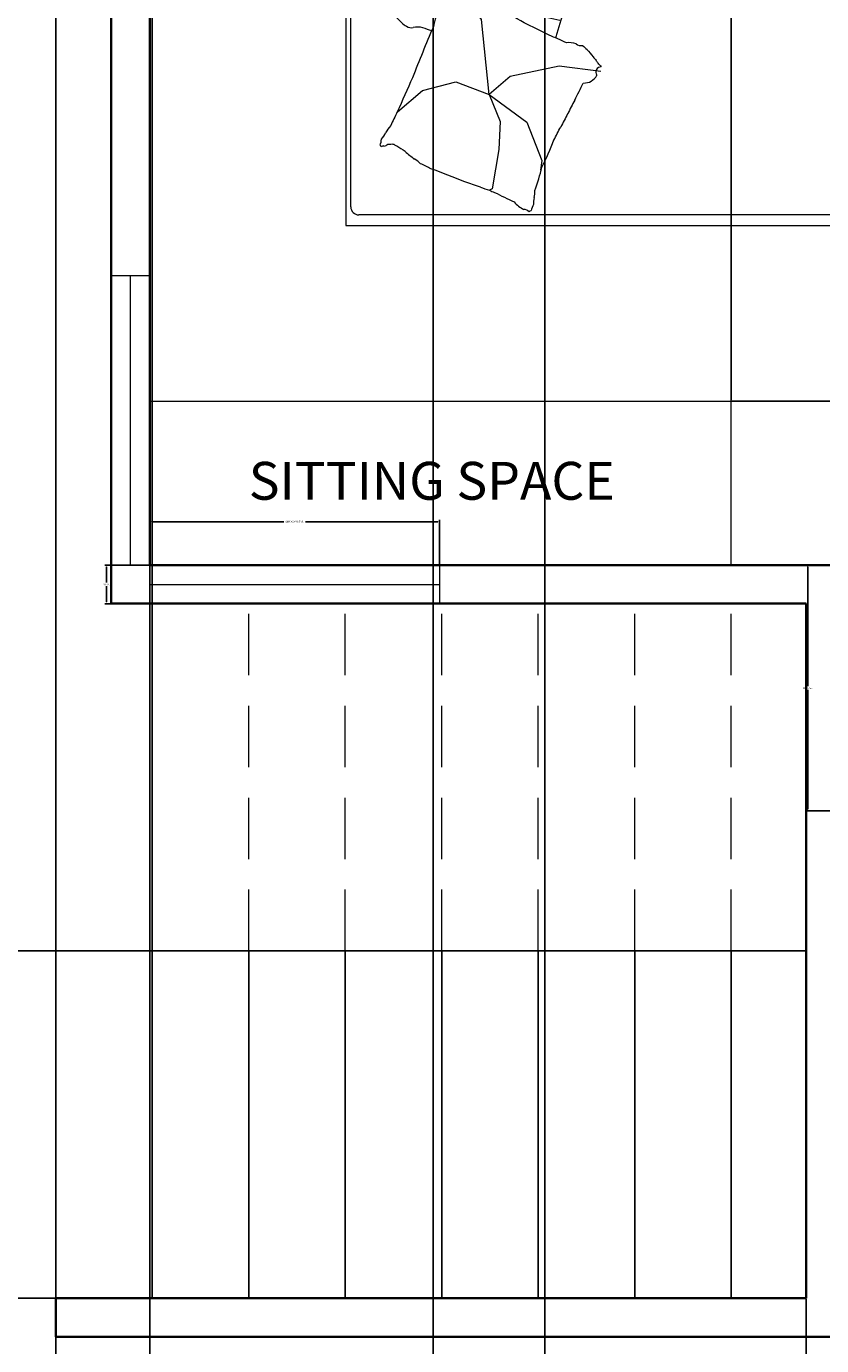
# Model space of a CAD drawing. Units: feet. Extents: x 1993 to 2298, y 2938 to 3641.
# Tile 3 of 11: x 2137 to 2219, y 3008 to 3144. Entities that reach past the tile are written whole.
import ezdxf

# ---------------------------------------------------------------- set-up
doc = ezdxf.new("R2010")
doc.units = ezdxf.units.FT
doc.linetypes.add('DASHED2', pattern=[9.525, 6.35, -3.175])
for name, color, linetype, lineweight in [('A-ANNO-DIMS', 2, 'Continuous', 18), ('A-AREA-IDEN', 7, 'Continuous', 18), ('A-FLOR-CASE', 8, 'Continuous', 18), ('A-FLOR-STRS', 7, 'Continuous', 25), ('A-FLOR-STRS-OVHD', 7, 'DASHED2', 13), ('A-GLAZ', 4, 'Continuous', 13), ('furniture', 8, 'Continuous', 18), ('WAL', 7, 'Continuous', 35)]:
    doc.layers.add(name, color=color, linetype=linetype, lineweight=lineweight)
doc.styles.add('DIM_FONT', font='SIMPLEX.shx', dxfattribs={"width": 0.8})
doc.styles.get("Standard").update_dxf_attribs({"font": 'arial.ttf'})
doc.dimstyles.get("Standard").update_dxf_attribs({"dimtxt": 0.18, "dimasz": 0.18, "dimexe": 0.18, "dimexo": 0.0625, "dimgap": 0.09, "dimtad": 0, "dimtih": 1, "dimtoh": 1, "dimdec": 4, "dimzin": 0, "dimdsep": 46, "dimtxsty": 'Standard', "dimcen": 0.09, "dimadec": 0, "dimazin": 0, "dimtfac": 1, "dimtdec": 4, "dimtofl": 0, "dimtmove": 0, "dimatfit": 3, "dimfxl": 1, "dimtolj": 1, "dimtzin": 0, "dimarcsym": 0})

# ---------------------------------------------------------------- blocks, each defined once
blk = doc.blocks.new('A$C79766A75')
for p, q in [((0.45, 1.9999), (0, 1.9999)), ((0, 1.9999), (0, 1.5499)), ((0.45, 1.5499), (0.45, 1.9999)), ((1.9506, 2), (0.4506, 2)), ((0.4506, 2), (0.4506, 0)), ((1.9506, 0), (1.9506, 2)), ((2.402, 1.9999), (1.952, 1.9999)), ((1.952, 1.9999), (1.952, 1.5499)), ((2.402, 1.5499), (2.402, 1.9999)), ((0.42, 1.9699), (0.03, 1.9699)), ((0.03, 1.9699), (0.03, 1.5799)), ((0.42, 1.5799), (0.42, 1.9699)), ((2.372, 1.9699), (1.982, 1.9699)), ((1.982, 1.9699), (1.982, 1.5799)), ((2.372, 1.5799), (2.372, 1.9699)), ((1.9506, 1.9476), (0.4506, 1.9476)), ((0.2304, 1.9125), (0.2304, 1.6061)), ((2.1824, 1.9125), (2.1824, 1.6061)), ((0.0743, 1.7595), (0.3834, 1.7595)), ((2.0263, 1.7595), (2.3354, 1.7595)), ((1.1461, 1.5617), (1.1254, 1.6443)), ((1.8553, 1.5617), (1.8346, 1.6443)), ((0.4234, 1.6034), (0.4228, 1.6034)), ((0.03, 1.5799), (0.42, 1.5799)), ((1.982, 1.5799), (2.372, 1.5799)), ((0, 1.5499), (0.45, 1.5499)), ((1.1536, 1.5317), (1.1461, 1.5617)), ((1.8628, 1.5317), (1.8553, 1.5617)), ((1.952, 1.5499), (2.402, 1.5499)), ((1.0972, 1.5115), (0.4791, 1.0841)), ((1.0972, 1.5115), (1.9048, 1.5115)), ((1.9248, 1.4915), (1.9248, 0.0322)), ((1.0383, 1.2184), (1.0246, 1.3138)), ((1.9048, 1.2389), (1.0354, 1.2389)), ((1.0365, 1.0883), (1.0383, 1.2184)), ((0.4791, 0.0622), (0.4791, 1.0841)), ((1.1731, 0.6316), (1.2523, 0.5276)), ((1.5696, 0.6317), (1.5559, 0.5286)), ((1.2523, 0.5276), (1.3274, 0.3973)), ((1.4223, 0.4407), (1.442, 0.5296)), ((1.5559, 0.5286), (1.5817, 0.4065)), ((1.6952, 0.4478), (1.7898, 0.4856)), ((1.7898, 0.4856), (1.8139, 0.4822)), ((1.4025, 0.3834), (1.4223, 0.4407)), ((1.6264, 0.355), (1.6952, 0.4478)), ((1.3274, 0.3973), (1.3452, 0.342)), ((1.5817, 0.4065), (1.6264, 0.355)), ((1.1139, 0.3597), (1.0779, 0.3397)), ((1.2167, 0.3736), (1.1139, 0.3597)), ((1.3452, 0.342), (1.2167, 0.3736)), ((1.3452, 0.342), (1.4025, 0.3834)), ((1.6264, 0.355), (1.6935, 0.3825)), ((1.6935, 0.3825), (1.7623, 0.379)), ((1.7623, 0.379), (1.8603, 0.3619)), ((1.8603, 0.3619), (1.8636, 0.3554)), ((1.2957, 0.2787), (1.3452, 0.342)), ((1.3452, 0.342), (1.3569, 0.2478)), ((1.4034, 0.3558), (1.3803, 0.2995)), ((1.4406, 0.3361), (1.3907, 0.3)), ((1.6264, 0.355), (1.4406, 0.3361)), ((1.5954, 0.2725), (1.6264, 0.355)), ((1.3803, 0.2995), (1.3626, 0.256)), ((1.3907, 0.3), (1.3787, 0.2914)), ((1.2305, 0.2313), (1.2957, 0.2787)), ((1.6161, 0.19), (1.5954, 0.2725)), ((1.1376, 0.2313), (1.2305, 0.2313)), ((1.3588, 0.2331), (1.3706, 0.1385)), ((1.6697, 0.1274), (1.6161, 0.19)), ((1.9048, 0.0122), (0.5291, 0.0122)), ((0.4506, 0), (1.9506, 0))]:
    blk.add_line(p, q)
for centre in [(0.2304, 1.7595), (2.1824, 1.7595)]:
    blk.add_circle(centre, 0.126)
for centre, radius, start, end in [((0.5232, 1.9139), 0.00342, 291.7883, 340.436), ((0.525, 1.9085), 0.00232, 340.436, 101.8931), ((0.5246, 1.9378), 0.0251, 274.3025, 291.7883), ((0.5311, 1.9093), 0.00428, 201.9904, 281.8931), ((0.5465, 1.8994), 0.0156, 158.579, 201.9904), ((0.5486, 1.9393), 0.0289, 239.3487, 274.3025), ((0.5458, 1.8568), 0.0539, 59.3487, 84.7408), ((0.546, 1.0829), 0.8208, 84.7408, 88.0921), ((0.6118, 2.0005), 0.0992, 254.0648, 274.2159), ((0.6775, 1.9817), 0.0992, 233.9136, 254.0648), ((0.6362, 0.406), 1.4943, 88.0921, 90.5757), ((0.7737, 2.1075), 0.234, 242.7604, 249.1397), ((0.7591, 1.0293), 0.8732, 90.5757, 94.8018), ((0.7631, 2.1919), 0.2897, 267.4614, 274.8018), ((0.8143, 2.0532), 0.1524, 259.8101, 267.4614), ((0.7515, 1.3747), 0.5293, 79.8101, 83.9133), ((1.1117, 1.6625), 0.2422, 97.5469, 105.744), ((1.0352, 2.2041), 0.3048, 278.4372, 285.744), ((1.1179, 2.0719), 0.1611, 270, 278.4372), ((1.1592, 2.0011), 0.0904, 258.7276, 270), ((1.1709, 1.9049), 0.0131, 153.4195, 258.7276), ((1.2325, 1.9139), 0.00342, 291.7883, 340.436), ((1.2342, 1.9085), 0.00232, 340.436, 101.8931), ((1.2338, 1.9378), 0.0251, 274.3025, 291.7883), ((1.2404, 1.9093), 0.00428, 201.9904, 281.8931), ((1.2558, 1.8994), 0.0156, 158.579, 201.9904), ((1.2578, 1.9393), 0.0289, 239.3487, 274.3025), ((1.2551, 1.8568), 0.0539, 59.3487, 84.7408), ((1.2552, 1.0829), 0.8208, 84.7408, 88.0921), ((1.3211, 2.0005), 0.0992, 254.0648, 274.2159), ((1.3868, 1.9817), 0.0992, 233.9136, 254.0648), ((1.3455, 0.406), 1.4943, 88.0921, 90.5757), ((1.4829, 2.1075), 0.234, 242.7604, 249.1397), ((1.4683, 1.0293), 0.8732, 90.5757, 94.8018), ((1.4724, 2.1919), 0.2897, 267.4614, 274.8018), ((1.5236, 2.0532), 0.1524, 259.8101, 267.4614), ((1.4607, 1.3747), 0.5293, 79.8101, 83.9133), ((1.821, 1.6625), 0.2422, 97.5469, 105.744), ((1.7444, 2.2041), 0.3048, 278.4372, 285.744), ((1.8271, 2.0719), 0.1611, 270, 278.4372), ((1.8684, 2.0011), 0.0904, 258.7276, 270), ((1.8802, 1.9049), 0.0131, 153.4195, 258.7276), ((0.4996, 1.8889), 0.0328, 338.579, 8.1335), ((0.2896, 1.8253), 0.246, 8.1335, 12.1095), ((0.7304, 1.9449), 0.0992, 216.1766, 233.9136), ((0.7661, 1.8961), 0.0992, 198.4397, 216.1766), ((0.738, 1.949), 0.0768, 231.6114, 242.7604), ((0.974, 2.1633), 0.3916, 226.1885, 231.6114), ((0.8451, 0.8466), 1.049, 83.9133, 90), ((1.046, 1.2129), 0.6827, 90, 97.5469), ((1.171, 1.8579), 0.0342, 94.4002, 153.4195), ((1.6324, 1.8735), 0.4918, 180, 186.2324), ((1.2088, 1.8889), 0.0328, 338.579, 8.1335), ((0.9988, 1.8253), 0.246, 8.1335, 12.1095), ((1.4396, 1.9449), 0.0992, 216.1766, 233.9136), ((1.4753, 1.8961), 0.0992, 198.4397, 216.1766), ((1.4473, 1.949), 0.0768, 231.6114, 242.7604), ((1.6833, 2.1633), 0.3916, 226.1885, 231.6114), ((1.5543, 0.8466), 1.049, 83.9133, 90), ((1.7552, 1.2129), 0.6827, 90, 97.5469), ((1.7511, 1.9723), 0.1399, 297.2036, 314.9024), ((1.8802, 1.8579), 0.0342, 94.4002, 153.4195), ((2.3416, 1.8735), 0.4918, 180, 186.2324), ((0.7297, 1.8867), 0.1983, 187.6809, 192.1095), ((1.4472, 1.8987), 0.9131, 183.3687, 187.6809), ((0.9057, 1.9982), 0.2252, 219.0349, 226.1885), ((0.7932, 1.8591), 0.0493, 208.3168, 219.0349), ((1.4389, 1.8867), 0.1983, 187.6809, 192.1095), ((2.1565, 1.8987), 0.9131, 183.3687, 187.6809), ((1.615, 1.9982), 0.2252, 219.0349, 226.1885), ((1.5025, 1.8591), 0.0493, 208.3168, 219.0349), ((1.6908, 1.9123), 0.1399, 314.9024, 332.6012), ((1.6887, 1.8881), 0.1511, 334.6449, 338.1851), ((1.7896, 1.8667), 0.0526, 318.5571, 334.6449), ((1.784, 1.9167), 0.0899, 306.2641, 318.5571), ((0.9392, 1.9062), 0.2002, 203.0028, 208.3168), ((1.3446, 1.7858), 0.204, 170.3156, 180), ((1.6484, 1.9062), 0.2002, 203.0028, 208.3168), ((1.6554, 1.8529), 0.1399, 332.6012, 343.485), ((1.7653, 1.8132), 0.0562, 341.2201, 0), ((1.6307, 1.8895), 0.2056, 338.1851, 341.2201), ((2.0538, 1.7858), 0.204, 170.3156, 180), ((1.2208, 1.7573), 0.6787, 178.3669, 183.3687), ((2.0027, 1.5994), 0.882, 167.8016, 170.3156), ((1.9301, 1.7573), 0.6787, 178.3669, 183.3687), ((1.6404, 1.8023), 0.1399, 343.485, 354.3689), ((1.73, 1.7719), 0.0915, 0, 14.6851), ((2.7119, 1.5994), 0.882, 167.8016, 170.3156), ((0.8192, 1.792), 0.3171, 347.8016, 351.9949), ((1.5284, 1.792), 0.3171, 347.8016, 351.9949), ((1.9066, 1.6447), 1.3652, 176.945, 178.3669), ((0.4711, 1.7556), 0.6588, 351.9949, 357.3351), ((2.6158, 1.6447), 1.3652, 176.945, 178.3669), ((1.1803, 1.7556), 0.6588, 351.9949, 357.3351), ((14.1519, 0.85), 13.6356, 176.49514, 176.94504), ((14.8612, 0.85), 13.6356, 176.49514, 176.94504), ((1.0578, 1.6474), 0.0677, 357.3351, 14.0452), ((1.767, 1.6474), 0.0677, 357.3351, 14.0452), ((0.7658, 2.8912), 1.4323, 294.3265, 296.4985), ((1.226, 2.0834), 0.5066, 290.6743, 294.3265), ((1.4305, 1.6796), 0.058, 274.0828, 290.6743), ((1.4679, 1.8969), 0.2721, 266.4448, 274.0828), ((0.8521, 1.5209), 0.3212, 170.0016, 176.4951), ((0.6583, 0.9067), 0.7387, 64.6889, 66.5156), ((0.7015, 0.888), 0.7387, 66.5156, 68.3423), ((1.5613, 1.5209), 0.3212, 170.0016, 176.4951), ((0.9025, 2.1618), 0.7286, 302.135, 305.8263), ((1.1895, 1.8508), 0.3126, 296.4985, 302.135), ((1.3675, 0.9067), 0.7387, 64.6889, 66.5156), ((1.4107, 0.888), 0.7387, 66.5156, 68.3423), ((0.513, 1.535), 0.0193, 350.0016, 16.6978), ((0.5822, 1.4654), 0.0767, 106.2212, 117.2841), ((0.5507, 1.5832), 0.0453, 282.869, 297.2841), ((0.5623, 1.6885), 0.1459, 273.574, 282.869), ((0.589, 2.7103), 1.164, 270.2865, 273.574), ((0.7584, 7.2662), 5.7185, 269.0296, 270.2865), ((0.9401, 4.9065), 3.3622, 267.3904, 269.0296), ((0.9811, 2.7573), 1.2165, 265.3824, 267.3904), ((0.8583, 0.139), 1.4048, 85.3824, 87.2509), ((1.0175, 1.3138), 0.2301, 87.2509, 101.5586), ((0.7501, 0.8688), 0.7387, 68.3423, 70.572), ((0.8043, 0.8497), 0.7387, 70.572, 72.8018), ((1.0449, 1.6886), 0.1459, 263.5659, 281.5586), ((1.1099, 1.6599), 0.1197, 252.6136, 263.5659), ((1.0587, 1.3144), 0.2297, 72.6136, 80.5159), ((1.2222, 1.535), 0.0193, 350.0016, 16.6978), ((1.2914, 1.4654), 0.0767, 106.2212, 117.2841), ((1.2599, 1.5832), 0.0453, 282.869, 297.2841), ((1.2716, 1.6885), 0.1459, 273.574, 282.869), ((1.2982, 2.7103), 1.164, 270.2865, 273.574), ((1.4677, 7.2662), 5.7185, 269.0296, 270.2865), ((1.6493, 4.9065), 3.3622, 267.3904, 269.0296), ((1.6903, 2.7573), 1.2165, 265.3824, 267.3904), ((1.5676, 0.139), 1.4048, 85.3824, 87.2509), ((1.7268, 1.3138), 0.2301, 87.2509, 101.5586), ((1.4594, 0.8688), 0.7387, 68.3423, 70.572), ((1.5136, 0.8497), 0.7387, 70.572, 72.8018), ((1.7541, 1.6886), 0.1459, 263.5659, 281.5586), ((1.8192, 1.6599), 0.1197, 252.6136, 263.5659), ((1.7679, 1.3144), 0.2297, 72.6136, 80.5159), ((0.5322, 1.5304), 0.00132, 16.6978, 97.1204), ((0.5579, 1.4467), 0.0875, 97.1204, 106.2212), ((0.745, 1.6407), 0.3751, 320.3555, 339.8512), ((1.108, 1.2635), 0.2708, 80.5159, 85.9171), ((1.1535, 1.5308), 0.000917, 85.9171, 194.0449), ((1.2414, 1.5304), 0.00132, 16.6978, 97.1204), ((1.2671, 1.4467), 0.0875, 97.1204, 106.2212), ((1.8172, 1.2635), 0.2708, 80.5159, 85.9171), ((1.8627, 1.5308), 0.000917, 85.9171, 194.0449), ((1.9048, 1.4915), 0.02, 0, 90), ((0.8556, 1.3759), 0.1801, 339.8512, 8.1356), ((1.9048, 1.2589), 0.02, 270, 0), ((-0.1888, 5.1029), 4.0646, 280.7276, 282.9255), ((0.7282, 1.1989), 0.0581, 262.2696, 280.7276), ((0.7833, 1.3309), 0.1942, 256.8096, 262.2696), ((0.2481, -1.3253), 2.5158, 76.8096, 78.3259), ((0.3953, -1.4284), 2.588, 78.3259, 80.505), ((-0.0248, 2.8487), 1.8351, 285.9352, 287.7364), ((0.3872, 1.7415), 0.6574, 282.9255, 285.9352), ((0.413, -2.64), 3.7801, 80.505, 82.308), ((1.1752, 0.6267), 0.0063, 166.7192, 233.4208), ((1.1734, 0.6272), 0.00443, 93.9484, 166.7192), ((1.163, 0.6103), 0.0142, 10.4074, 53.4208), ((1.1755, 0.5964), 0.0352, 69.6548, 93.9484), ((1.1669, 0.5731), 0.0601, 51.4146, 69.6548), ((1.7751, 0.3162), 0.3825, 126.2163, 127.5287), ((1.5806, 0.5924), 0.0452, 127.5287, 134.1274), ((1.5093, 0.6825), 0.0697, 308.8136, 314.1274), ((1.5706, 0.6318), 0.0127, 176.7545, 308.8136), ((1.5621, 0.59), 0.0359, 356.7545, 62.7098), ((0.8605, 0.749), 0.352, 329.0944, 333.1821), ((1.1396, 0.6079), 0.0393, 333.1821, 345.4291), ((1.1011, 0.5989), 0.0771, 2.7286, 10.4074), ((1.1628, 0.6019), 0.0153, 345.4291, 2.7286), ((1.2538, 0.682), 0.0792, 231.4146, 247.2931), ((1.5463, 1.3811), 0.8371, 247.2931, 249.8713), ((3.0113, 5.3783), 5.0942, 249.8713, 250.9164), ((1.4519, 0.6426), 0.0774, 313.5224, 324.1064), ((1.383, 0.7705), 0.2176, 307.2151, 313.5224), ((1.1426, 1.1456), 0.6605, 306.2163, 307.2151), ((0.9961, 0.6678), 0.194, 320.2995, 329.0944), ((2.374, 3.5362), 3.145, 250.9164, 253.3915), ((1.5435, 0.5526), 0.0458, 157.5838, 188.0492), ((1.4828, 0.5833), 0.0226, 324.1064, 8.0492), ((0.2201, -2.1858), 3.0972, 62.7098, 63.5853), ((2.5711, 2.3551), 2.0162, 242.5001, 243.5853), ((1.3115, 0.4414), 0.1965, 153.9265, 162.1604), ((1.2077, 0.4922), 0.081, 140.2995, 153.9265), ((2.4089, 0.1204), 1.0054, 154.9471, 157.5838), ((4.5245, 5.9445), 6.1019, 242.15178, 242.50014), ((-0.9881, -4.647), 5.8383, 62.15178, 62.50792), ((3.0311, -0.112), 2.003, 162.1604, 164.7375), ((2.9813, -0.2643), 1.6868, 152.9116, 154.9471), ((1.5084, 0.6341), 0.1166, 253.3915, 259.2634), ((1.5182, -0.068), 0.6236, 62.5079, 69.2514), ((1.7121, 0.0657), 0.43, 69.2514, 77.3748), ((1.8682, 0.4049), 0.063, 77.3748, 93.3881), ((1.8955, 0.5247), 0.0599, 256.9598, 273.3881), ((1.9257, 0.5082), 0.0509, 238.3083, 256.9598), ((1.9201, 0.4587), 0.0058, 180.9614, 238.3083), ((2.8096, -0.3311), 1.5652, 150.064, 152.9116), ((1.8435, 0.4743), 0.0755, 310.5086, 333.6668), ((1.9279, 0.441), 0.0168, 130.5086, 180.9614), ((2.6887, -0.0186), 1.6481, 164.7375, 166.159), ((-0.5166, 1.5491), 2.6619, 333.6668, 334.8268), ((0.5589, 0.5062), 0.5454, 343.6878, 346.159), ((1.2176, 0.4627), 0.2143, 330.064, 337.7645), ((1.701, 0.4319), 0.1798, 334.8268, 339.2919), ((-1.4109, 1.284), 2.6619, 338.0627, 339.2227), ((0.9098, 0.4035), 0.1798, 339.2227, 343.6878), ((3.4079, -0.2212), 1.6481, 160.3416, 161.7631), ((1.3456, 0.5261), 0.5454, 339.2919, 341.7631), ((3.6966, -0.4634), 2.003, 157.7645, 160.3416), ((1.0533, 0.2524), 0.0168, 134.9045, 185.3572), ((0.9882, 0.3177), 0.0755, 314.9045, 338.0627), ((1.0424, 0.2513), 0.0058, 185.3572, 242.7041), ((1.0631, 0.2914), 0.0509, 242.7041, 261.3557), ((1.0645, 0.3003), 0.0599, 261.3557, 277.784), ((1.0811, 0.1786), 0.063, 81.7707, 97.784), ((1.0286, -0.1846), 0.43, 73.6473, 81.7707), ((1.3465, 0.2383), 0.00467, 287.1867, 70.6201), ((1.3486, 0.2247), 0.0092, 70.6201, 94.2593), ((1.3694, 0.234), 0.0231, 107.1867, 157.7645), ((1.3563, 0.267), 0.034, 262.0178, 274.2593), ((1.4091, 0.4221), 0.1955, 255.1193, 262.0178), ((0.974, -0.3705), 0.6236, 66.9038, 73.6473), ((-1.0716, -5.1672), 5.8383, 66.54766, 66.9038), ((1.358, 0.0507), 0.1794, 75.1193, 82.3216), ((1.4096, 0.153), 0.0712, 82.3216, 94.5118), ((1.4285, 0.2893), 0.0663, 261.8784, 274.5118), ((1.4755, 0.332), 0.1166, 248.9957, 261.8784), ((2.7121, 3.1012), 3.145, 246.5205, 248.9957), ((2.4175, -0.1202), 1.0054, 160.6552, 161.9797), ((1.9797, 0.1108), 0.1965, 149.5306, 157.7645), ((3.6805, 5.7866), 6.1019, 246.54766, 246.89602), ((2.0773, 2.0287), 2.0162, 246.896, 247.9812), ((1.4382, 0.1619), 0.0226, 328.5023, 12.4451), ((1.505, 0.1766), 0.0458, 161.9797, 192.4451), ((3.6993, 4.7998), 5.0942, 245.4754, 246.5205), ((1.6279, 0.2819), 0.194, 315.9036, 324.6985), ((1.856, 0.1288), 0.081, 135.9036, 149.5306), ((0.1602, -2.7118), 3.0972, 67.1056, 67.9812), ((1.3512, 0.1084), 0.0359, 1.1504, 67.1056), ((1.2874, 0.2845), 0.2176, 311.611, 317.9183), ((1.3914, 0.1905), 0.0774, 317.9183, 328.5023), ((1.4661, 0.3294), 0.352, 324.6985, 328.7862), ((1.3997, 0.1094), 0.0127, 181.1504, 313.2095), ((1.3607, 0.1509), 0.0697, 313.2095, 318.5233), ((1.4468, 0.0748), 0.0452, 131.9246, 138.5233), ((1.6722, -0.1762), 0.3825, 130.6122, 131.9246), ((0.9933, 0.6156), 0.6605, 310.6122, 311.611), ((2.051, 0.8725), 0.8371, 242.8972, 245.4754), ((1.7576, 0.1689), 0.0792, 227.0187, 242.8972), ((1.6963, 0.0438), 0.0601, 47.0187, 65.2589), ((1.7345, 0.1188), 0.0153, 341.0332, 358.3327), ((1.6723, 0.1058), 0.0771, 358.3327, 6.0115), ((1.7401, 0.0928), 0.0142, 6.0115, 49.0249), ((1.7162, 0.1388), 0.0393, 328.7862, 341.0332), ((1.737, 0.0526), 0.0352, 65.2589, 89.5525), ((1.756, 0.0832), 0.00443, 89.5525, 162.3233), ((1.7602, 0.0924), 0.0063, 162.3233, 229.0249), ((0.5291, 0.0622), 0.05, 180, 270), ((1.9048, 0.0322), 0.02, 270, 0)]:
    blk.add_arc(centre, radius, start, end)
at = {"style": 'DIM_FONT', "text_generation_flag": 4, "width": 0.8, "flags": 9}
for tag in ['XSIZE', 'YSIZE']:
    blk.add_attdef(tag, (1.9506, 2), '', height=0.0005, rotation=180, dxfattribs=at)
blk = doc.blocks.new('WIN-2FT6')
for p, q in [((0, 4), (0, 0)), ((30, 4), (30, 0)), ((0, 2), (30, 2))]:
    blk.add_line(p, q)
blk = doc.blocks.new('*D28')
at = {"layer": 'A-ANNO-DIMS', "color": 0, "lineweight": -2, "transparency": 16777216}
for p, q in [((2221.7, 3088.53), (2217.75, 3088.53)), ((2217.93, 3088.35), (2217.93, 3075.97)), ((2217.93, 3063.22), (2217.93, 3075.6)), ((2221.7, 3063.04), (2217.75, 3063.04))]:
    blk.add_line(p, q, dxfattribs=at)
at = {"layer": 'A-ANNO-DIMS', "color": 0, "transparency": 16777216}
for points in [[(2217.9, 3088.35), (2217.96, 3088.35), (2217.93, 3088.53)], [(2217.9, 3063.22), (2217.96, 3063.22), (2217.93, 3063.04)]]:
    blk.add_solid(points, dxfattribs=at)
at = {"layer": 'Defpoints', "color": 0, "transparency": 16777216}
for p in [(2221.76, 3088.53), (2217.93, 3063.04), (2221.76, 3063.04)]:
    blk.add_point(p, dxfattribs=at)
at = {"layer": 'A-ANNO-DIMS', "color": 0, "transparency": 16777216, "insert": (2217.93, 3075.78), "char_height": 0.18, "attachment_point": 5}
blk.add_mtext('\\A1;DOOR 25', dxfattribs=at)
blk = doc.blocks.new('*D38')
at = {"layer": 'A-ANNO-DIMS', "color": 0, "lineweight": -2, "transparency": 16777216}
for p, q in [((2149.76, 3088.6), (2149.76, 3093.21)), ((2149.94, 3093.03), (2163.64, 3093.03)), ((2179.58, 3093.03), (2165.88, 3093.03)), ((2179.76, 3088.6), (2179.76, 3093.21))]:
    blk.add_line(p, q, dxfattribs=at)
at = {"layer": 'A-ANNO-DIMS', "color": 0, "transparency": 16777216}
for points in [[(2149.94, 3093.06), (2149.94, 3093), (2149.76, 3093.03)], [(2179.58, 3093.06), (2179.58, 3093), (2179.76, 3093.03)]]:
    blk.add_solid(points, dxfattribs=at)
at = {"layer": 'Defpoints', "color": 0, "transparency": 16777216}
for p in [(2179.76, 3093.03), (2149.76, 3088.53), (2179.76, 3088.53)]:
    blk.add_point(p, dxfattribs=at)
at = {"layer": 'A-ANNO-DIMS', "color": 0, "transparency": 16777216, "insert": (2164.76, 3093.03), "char_height": 0.18, "attachment_point": 5}
blk.add_mtext('\\A1;WINDOW 30 TYP.', dxfattribs=at)
blk = doc.blocks.new('*D39')
at = {"layer": 'A-ANNO-DIMS', "color": 0, "lineweight": -2, "transparency": 16777216}
for p, q in [((2149.7, 3088.53), (2145.08, 3088.53)), ((2145.26, 3088.35), (2145.26, 3086.71)), ((2145.26, 3084.71), (2145.26, 3086.35)), ((2149.7, 3084.53), (2145.08, 3084.53))]:
    blk.add_line(p, q, dxfattribs=at)
at = {"layer": 'A-ANNO-DIMS', "color": 0, "transparency": 16777216}
for points in [[(2145.23, 3088.35), (2145.29, 3088.35), (2145.26, 3088.53)], [(2145.23, 3084.71), (2145.29, 3084.71), (2145.26, 3084.53)]]:
    blk.add_solid(points, dxfattribs=at)
at = {"layer": 'Defpoints', "color": 0, "transparency": 16777216}
for p in [(2145.26, 3088.53), (2149.76, 3088.53), (2149.76, 3084.53)]:
    blk.add_point(p, dxfattribs=at)
at = {"layer": 'A-ANNO-DIMS', "color": 0, "transparency": 16777216, "insert": (2145.26, 3086.53), "char_height": 0.18, "attachment_point": 5}
blk.add_mtext('\\A1;4 TYP.', dxfattribs=at)
blk = doc.blocks.new('*D58')
at = {"layer": 'A-ANNO-DIMS', "color": 0, "lineweight": -2, "transparency": 16777216}
for p, q in [((2139.94, 3048.53), (1993.61, 3048.53)), ((1993.79, 3048.35), (1993.79, 3030.72)), ((1993.79, 3012.71), (1993.79, 3030.35)), ((2139.94, 3012.53), (1993.61, 3012.53))]:
    blk.add_line(p, q, dxfattribs=at)
at = {"layer": 'A-ANNO-DIMS', "color": 0, "transparency": 16777216}
for points in [[(1993.76, 3048.35), (1993.82, 3048.35), (1993.79, 3048.53)], [(1993.76, 3012.71), (1993.82, 3012.71), (1993.79, 3012.53)]]:
    blk.add_solid(points, dxfattribs=at)
at = {"layer": 'Defpoints', "color": 0, "transparency": 16777216}
for p in [(1993.79, 3048.53), (2140, 3048.53), (2140, 3012.53)]:
    blk.add_point(p, dxfattribs=at)
at = {"layer": 'A-ANNO-DIMS', "color": 0, "transparency": 16777216, "insert": (1993.79, 3030.53), "char_height": 0.18, "attachment_point": 5}
blk.add_mtext('\\A1;36', dxfattribs=at)
blk = doc.blocks.new('*D59')
at = {"layer": 'A-ANNO-DIMS', "color": 0, "lineweight": -2, "transparency": 16777216}
for p, q in [((2140, 3048.6), (2140, 3640.68)), ((2150, 3048.6), (2150, 3640.68)), ((2140.18, 3640.5), (2144.79, 3640.5)), ((2149.82, 3640.5), (2145.21, 3640.5))]:
    blk.add_line(p, q, dxfattribs=at)
at = {"layer": 'A-ANNO-DIMS', "color": 0, "transparency": 16777216}
for points in [[(2140.18, 3640.53), (2140.18, 3640.47), (2140, 3640.5)], [(2149.82, 3640.53), (2149.82, 3640.47), (2150, 3640.5)]]:
    blk.add_solid(points, dxfattribs=at)
at = {"layer": 'Defpoints', "color": 0, "transparency": 16777216}
for p in [(2150, 3640.5), (2140, 3048.53), (2150, 3048.53)]:
    blk.add_point(p, dxfattribs=at)
at = {"layer": 'A-ANNO-DIMS', "color": 0, "transparency": 16777216, "insert": (2145, 3640.5), "char_height": 0.18, "attachment_point": 5}
blk.add_mtext('\\A1;10', dxfattribs=at)
blk = doc.blocks.new('*D60')
at = {"layer": 'A-ANNO-DIMS', "color": 0, "lineweight": -2, "transparency": 16777216}
for p, q in [((2140, 3012.47), (2140, 2937.86)), ((2217.76, 3012.47), (2217.76, 2937.86)), ((2140.18, 2938.03), (2178.49, 2938.03)), ((2217.58, 2938.03), (2179.27, 2938.03))]:
    blk.add_line(p, q, dxfattribs=at)
at = {"layer": 'A-ANNO-DIMS', "color": 0, "transparency": 16777216}
for points in [[(2140.18, 2938.07), (2140.18, 2938.01), (2140, 2938.03)], [(2217.58, 2938.07), (2217.58, 2938.01), (2217.76, 2938.03)]]:
    blk.add_solid(points, dxfattribs=at)
at = {"layer": 'Defpoints', "color": 0, "transparency": 16777216}
for p in [(2140, 3012.53), (2217.76, 3012.53), (2217.76, 2938.03)]:
    blk.add_point(p, dxfattribs=at)
at = {"layer": 'A-ANNO-DIMS', "color": 0, "transparency": 16777216, "insert": (2178.88, 2938.03), "char_height": 0.18, "attachment_point": 5}
blk.add_mtext('\\A1;77.76', dxfattribs=at)
blk = doc.blocks.new('*D65')
at = {"layer": 'A-ANNO-DIMS', "color": 0, "lineweight": -2, "transparency": 16777216}
for p, q in [((2179.12, 3231.85), (2179.12, 2937.86)), ((2149.76, 3228.47), (2149.76, 2937.86)), ((2149.94, 2938.03), (2164.04, 2938.03)), ((2178.94, 2938.03), (2164.83, 2938.03))]:
    blk.add_line(p, q, dxfattribs=at)
at = {"layer": 'A-ANNO-DIMS', "color": 0, "transparency": 16777216}
for points in [[(2149.94, 2938.07), (2149.94, 2938.01), (2149.76, 2938.03)], [(2178.94, 2938.07), (2178.94, 2938.01), (2179.12, 2938.03)]]:
    blk.add_solid(points, dxfattribs=at)
at = {"layer": 'Defpoints', "color": 0, "transparency": 16777216}
for p in [(2179.12, 3231.92), (2149.76, 3228.53), (2179.12, 2938.03)]:
    blk.add_point(p, dxfattribs=at)
at = {"layer": 'A-ANNO-DIMS', "color": 0, "transparency": 16777216, "insert": (2164.44, 2938.03), "char_height": 0.18, "attachment_point": 5}
blk.add_mtext('\\A1;29.36', dxfattribs=at)
blk = doc.blocks.new('*D69')
at = {"layer": 'A-ANNO-DIMS', "color": 0, "lineweight": -2, "transparency": 16777216}
for p, q in [((2149.76, 3492.27), (2149.76, 2937.86)), ((2190.69, 3492.27), (2190.69, 2937.86)), ((2149.94, 2938.03), (2169.83, 2938.03)), ((2190.51, 2938.03), (2170.62, 2938.03))]:
    blk.add_line(p, q, dxfattribs=at)
at = {"layer": 'A-ANNO-DIMS', "color": 0, "transparency": 16777216}
for points in [[(2149.94, 2938.07), (2149.94, 2938.01), (2149.76, 2938.03)], [(2190.51, 2938.07), (2190.51, 2938.01), (2190.69, 2938.03)]]:
    blk.add_solid(points, dxfattribs=at)
at = {"layer": 'Defpoints', "color": 0, "transparency": 16777216}
for p in [(2149.76, 3492.33), (2190.69, 3492.33), (2190.69, 2938.03)]:
    blk.add_point(p, dxfattribs=at)
at = {"layer": 'A-ANNO-DIMS', "color": 0, "transparency": 16777216, "insert": (2170.23, 2938.03), "char_height": 0.18, "attachment_point": 5}
blk.add_mtext('\\A1;40.93', dxfattribs=at)
blk = doc.blocks.new('*D73')
at = {"layer": 'A-ANNO-DIMS', "color": 0, "lineweight": -2, "transparency": 16777216}
for p, q in [((2149.76, 3105.6), (2149.76, 3640.68)), ((2210, 3105.6), (2210, 3640.68)), ((2149.94, 3640.5), (2179.49, 3640.5)), ((2209.82, 3640.5), (2180.27, 3640.5))]:
    blk.add_line(p, q, dxfattribs=at)
at = {"layer": 'A-ANNO-DIMS', "color": 0, "transparency": 16777216}
for points in [[(2149.94, 3640.53), (2149.94, 3640.47), (2149.76, 3640.5)], [(2209.82, 3640.53), (2209.82, 3640.47), (2210, 3640.5)]]:
    blk.add_solid(points, dxfattribs=at)
at = {"layer": 'Defpoints', "color": 0, "transparency": 16777216}
for p in [(2210, 3640.5), (2149.76, 3105.53), (2210, 3105.53)]:
    blk.add_point(p, dxfattribs=at)
at = {"layer": 'A-ANNO-DIMS', "color": 0, "transparency": 16777216, "insert": (2179.88, 3640.5), "char_height": 0.18, "attachment_point": 5}
blk.add_mtext('\\A1;60.24', dxfattribs=at)
blk = doc.blocks.new('*D74')
at = {"layer": 'A-ANNO-DIMS', "color": 0, "lineweight": -2, "transparency": 16777216}
for p, q in [((2210.06, 3105.53), (2242.15, 3105.53)), ((2241.97, 3105.35), (2241.97, 3097.21)), ((2241.97, 3088.71), (2241.97, 3096.85)), ((2210.06, 3088.53), (2242.15, 3088.53))]:
    blk.add_line(p, q, dxfattribs=at)
at = {"layer": 'A-ANNO-DIMS', "color": 0, "transparency": 16777216}
for points in [[(2241.94, 3105.35), (2242, 3105.35), (2241.97, 3105.53)], [(2241.94, 3088.71), (2242, 3088.71), (2241.97, 3088.53)]]:
    blk.add_solid(points, dxfattribs=at)
at = {"layer": 'Defpoints', "color": 0, "transparency": 16777216}
for p in [(2210, 3105.53), (2210, 3088.53), (2241.97, 3088.53)]:
    blk.add_point(p, dxfattribs=at)
at = {"layer": 'A-ANNO-DIMS', "color": 0, "transparency": 16777216, "insert": (2241.97, 3097.03), "char_height": 0.18, "attachment_point": 5}
blk.add_mtext('\\A1;17', dxfattribs=at)
blk = doc.blocks.new('*D75')
at = {"layer": 'A-ANNO-DIMS', "color": 0, "lineweight": -2, "transparency": 16777216}
for p, q in [((2029.76, 3008.6), (2029.76, 3640.68)), ((2140, 3008.6), (2140, 3640.68)), ((2029.94, 3640.5), (2084.42, 3640.5)), ((2139.82, 3640.5), (2085.33, 3640.5))]:
    blk.add_line(p, q, dxfattribs=at)
at = {"layer": 'A-ANNO-DIMS', "color": 0, "transparency": 16777216}
for points in [[(2029.94, 3640.53), (2029.94, 3640.47), (2029.76, 3640.5)], [(2139.82, 3640.53), (2139.82, 3640.47), (2140, 3640.5)]]:
    blk.add_solid(points, dxfattribs=at)
at = {"layer": 'Defpoints', "color": 0, "transparency": 16777216}
for p in [(2140, 3640.5), (2029.76, 3008.53), (2140, 3008.53)]:
    blk.add_point(p, dxfattribs=at)
at = {"layer": 'A-ANNO-DIMS', "color": 0, "transparency": 16777216, "insert": (2084.88, 3640.5), "char_height": 0.18, "attachment_point": 5}
blk.add_mtext('\\A1;110.24', dxfattribs=at)

msp = doc.modelspace()

# ---------------------------------------------------------------- linework, layer by layer
at = {"layer": 'A-FLOR-CASE'}
for p in [(2149.7583, 3105.5338), (2210, 3088.5338)]:
    msp.add_line(p, (2210, 3105.5338), dxfattribs=at)
at = {"layer": 'A-FLOR-STRS'}
for p, q in [((2217.7583, 3048.5338), (2140, 3048.5338)), ((2140, 3048.5338), (2140, 3010.5338)), ((2150, 3048.5338), (2150, 3012.5338)), ((2160, 3048.5338), (2160, 3012.5338)), ((2170, 3048.5338), (2170, 3012.5338)), ((2180, 3048.5338), (2180, 3012.5338)), ((2190, 3048.5338), (2190, 3012.5338)), ((2200, 3048.5338), (2200, 3012.5338)), ((2210, 3048.5338), (2210, 3012.5338))]:
    msp.add_line(p, q, dxfattribs=at)
at = {"layer": 'A-FLOR-STRS-OVHD'}
for p, q in [((2150, 3048.5338), (2150, 3084.5338)), ((2160, 3048.5338), (2160, 3084.5338)), ((2170, 3048.5338), (2170, 3084.5338)), ((2180, 3048.5338), (2180, 3084.5338)), ((2190, 3048.5338), (2190, 3084.5338)), ((2200, 3048.5338), (2200, 3084.5338)), ((2210, 3048.5338), (2210, 3084.5338))]:
    msp.add_line(p, q, dxfattribs=at)
at = {"layer": 'WAL'}
for p, q in [((2145.7583, 3084.5338), (2145.7583, 3292.5338)), ((2149.7583, 3088.5338), (2149.7583, 3224.5338)), ((2149.7583, 3088.5338), (2221.7583, 3088.5338)), ((2145.7583, 3084.5338), (2217.7583, 3084.5338)), ((2217.7583, 3084.5338), (2217.7583, 3012.5338)), ((2217.7583, 3012.5338), (2140, 3012.5338)), ((2140, 3012.5338), (2140, 3008.5338)), ((2265.7583, 3008.5338), (2140, 3008.5338))]:
    msp.add_line(p, q, dxfattribs=at)

# ---------------------------------------------------------------- block references
at = {"layer": 'A-GLAZ', "rotation": 90.00000000000003}
msp.add_blockref('WIN-2FT6', (2149.7581, 3088.5335), dxfattribs=at)
at = {"layer": 'A-GLAZ'}
msp.add_blockref('WIN-2FT6', (2149.758, 3084.534), dxfattribs=at)
at = {"layer": 'furniture', "xscale": 41.83725109546206, "yscale": 41.83725109546206, "zscale": 41.83725109546206, "rotation": 270}
msp.add_blockref('A$C79766A75', (2170.0686, 3205.3572), dxfattribs=at)

# ---------------------------------------------------------------- texts
at = {"layer": 'A-AREA-IDEN'}
msp.add_text('SITTING SPACE', height=3.928054, dxfattribs=at).set_placement((2160, 3095.3045))

# ---------------------------------------------------------------- dimensions: what is measured, and where the dimension line sits
at = {"layer": 'A-ANNO-DIMS'}
for base, p1, p2, override, picture, middle in [((2140, 3640.4988), (2029.7583, 3008.5338), (2140, 3008.5338), {"dimdec": 2, "dimlfac": 1, "dimrnd": 0, "dimzin": 0, "dimdsep": 46, "dimlunit": 2}, '*D75', (2084.8792, 3640.4988)), ((2150, 3640.4988), (2140, 3048.5338), (2150, 3048.5338), {"dimdec": 0, "dimlfac": 1, "dimrnd": 0, "dimzin": 0, "dimdsep": 46, "dimlunit": 2}, '*D59', (2145, 3640.4988)), ((2210, 3640.4988), (2149.7583, 3105.5338), (2210, 3105.5338), {"dimdec": 2, "dimlfac": 1, "dimrnd": 0, "dimzin": 0, "dimdsep": 46, "dimlunit": 2}, '*D73', (2179.8792, 3640.4988)), ((2190.6917, 2938.035), (2149.7583, 3492.3338), (2190.6917, 3492.3338), {"dimdec": 2, "dimlfac": 1, "dimrnd": 0, "dimzin": 0, "dimdsep": 46, "dimlunit": 2}, '*D69', (2170.225, 2938.035)), ((2179.1188, 2938.035), (2149.7583, 3228.5338), (2179.1188, 3231.9167), {"dimdec": 2, "dimlfac": 1, "dimrnd": 0, "dimzin": 0, "dimdsep": 46, "dimlunit": 2}, '*D65', (2164.4386, 2938.035)), ((2217.7583, 2938.035), (2140, 3012.5338), (2217.7583, 3012.5338), {"dimdec": 2, "dimlfac": 1, "dimrnd": 0, "dimzin": 0, "dimdsep": 46, "dimlunit": 2}, '*D60', (2178.8792, 2938.035))]:
    dim = msp.add_linear_dim(base=base, p1=p1, p2=p2, dimstyle='Standard', override=override, dxfattribs=at)
    dim.commit()
    dim.dimension.update_dxf_attribs({"geometry": picture, "text_midpoint": middle})
for base, p1, p2, angle, picture, middle in [((2241.965, 3088.5338), (2210, 3105.5338), (2210, 3088.5338), 270, '*D74', (2241.965, 3097.0338)), ((1993.7933, 3048.5338), (2140, 3012.5338), (2140, 3048.5338), 90, '*D58', (1993.7933, 3030.5338))]:
    dim = msp.add_linear_dim(base=base, p1=p1, p2=p2, angle=angle, dimstyle='Standard', override={"dimdec": 0, "dimlfac": 1, "dimrnd": 0, "dimzin": 0, "dimdsep": 46, "dimlunit": 2}, dxfattribs=at)
    dim.commit()
    dim.dimension.update_dxf_attribs({"geometry": picture, "text_midpoint": middle})
dim = msp.add_linear_dim(base=(2179.7583, 3093.0338), p1=(2149.7583, 3088.5338), p2=(2179.7583, 3088.5338), text='WINDOW <> TYP.', dimstyle='Standard', override={"dimdec": 0, "dimlfac": 1, "dimrnd": 0, "dimzin": 0, "dimdsep": 46, "dimlunit": 2}, dxfattribs=at)
dim.commit()
dim.dimension.update_dxf_attribs({"geometry": '*D38', "text_midpoint": (2164.7583, 3093.0338)})
for base, p1, p2, angle, text, picture, middle in [((2145.2583, 3088.5338), (2149.7583, 3084.5338), (2149.7583, 3088.5338), 90, '<> TYP.', '*D39', (2145.2583, 3086.5338)), ((2217.9337, 3063.0362), (2221.7583, 3088.5338), (2221.7583, 3063.0362), 270, 'DOOR <>', '*D28', (2217.9337, 3075.785))]:
    dim = msp.add_linear_dim(base=base, p1=p1, p2=p2, angle=angle, text=text, dimstyle='Standard', override={"dimdec": 0, "dimlfac": 1, "dimrnd": 0, "dimzin": 0, "dimdsep": 46, "dimlunit": 2}, dxfattribs=at)
    dim.commit()
    dim.dimension.update_dxf_attribs({"geometry": picture, "text_midpoint": middle})

doc.saveas('drawing.dxf')
